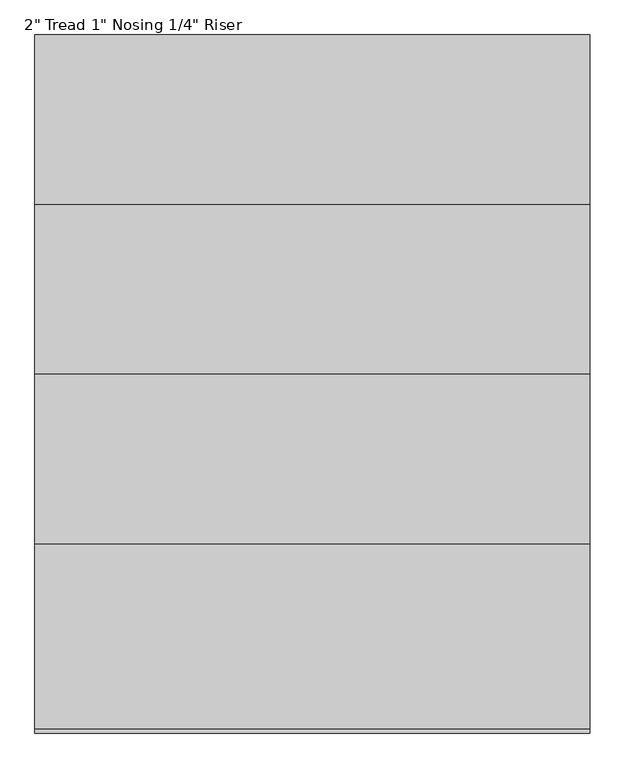
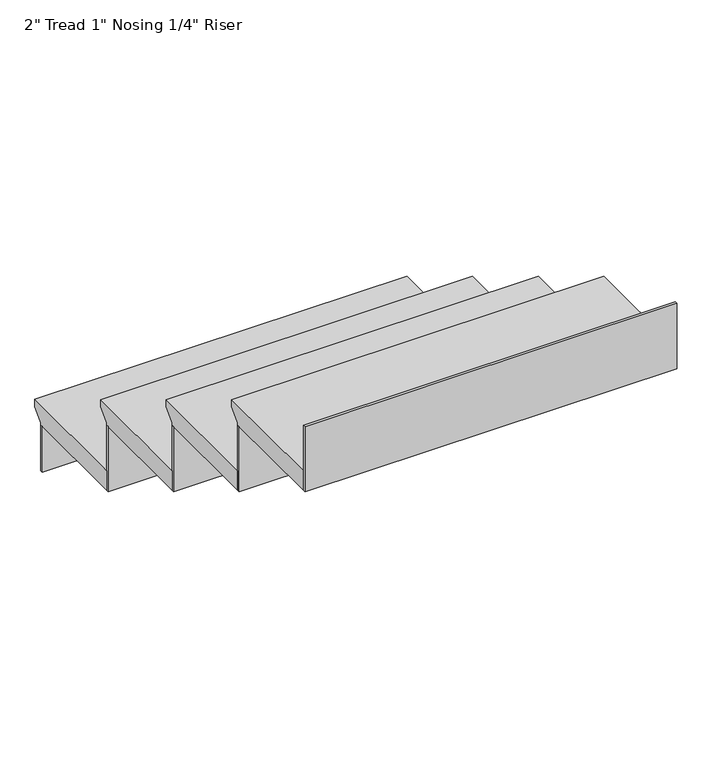
"""IFC4 building model written with IfcOpenShell, lengths in millimetres: stair flight geometry."""

from ifc_helpers import new_model, si_unit, frame, origin, place, context, project, spatial, polyline, outline, extrude, source, transform, mapped, element, save


def stair_flight_987ae6dc(model_context):
    return source(origin(), model_context, "Body", "SweptSolid", [
        extrude(outline(polyline([(618.7061342, 1693.3333333), (923.5061342, 1693.3333333), (923.5061342, 1674.2833333), (898.1061342, 1648.8833333), (898.1061342, 1642.5333333), (618.7061342, 1642.5333333), (618.7061342, 1693.3333333)])), frame((-4563.8448749, 0.0, 0.0), z_axis=(1.0, 0.0, 0.0), x_axis=(0.0, 1.0, 0.0)), (0.0, 0.0, 1.0), 914.4),
        extrude(outline(polyline([(-4563.8448749, 891.7561342), (-4563.8448749, 898.1061342), (-3649.4448749, 898.1061342), (-3649.4448749, 891.7561342), (-4563.8448749, 891.7561342)])), frame((0.0, 0.0, 1524.0), z_axis=(0.0, 0.0, 1.0), x_axis=(1.0, 0.0, 0.0)), (0.0, 0.0, 1.0), 118.5333333),
        extrude(outline(polyline([(-4563.8448749, 612.3561342), (-4563.8448749, 618.7061342), (-3649.4448749, 618.7061342), (-3649.4448749, 612.3561342), (-4563.8448749, 612.3561342)])), frame((0.0, 0.0, 1642.5333333), z_axis=(0.0, 0.0, 1.0), x_axis=(1.0, 0.0, 0.0)), (0.0, 0.0, 1.0), 169.3333333),
        extrude(outline(polyline([(339.3061342, 1862.6666667), (644.1061342, 1862.6666667), (644.1061342, 1843.6166667), (618.7061342, 1818.2166667), (618.7061342, 1811.8666667), (339.3061342, 1811.8666667), (339.3061342, 1862.6666667)])), frame((-4563.8448749, 0.0, 0.0), z_axis=(1.0, 0.0, 0.0), x_axis=(0.0, 1.0, 0.0)), (0.0, 0.0, 1.0), 914.4),
        extrude(outline(polyline([(-4563.8448749, 332.9561342), (-4563.8448749, 339.3061342), (-3649.4448749, 339.3061342), (-3649.4448749, 332.9561342), (-4563.8448749, 332.9561342)])), frame((0.0, 0.0, 1811.8666667), z_axis=(0.0, 0.0, 1.0), x_axis=(1.0, 0.0, 0.0)), (0.0, 0.0, 1.0), 169.3333333),
        extrude(outline(polyline([(59.9061342, 2032.0), (364.7061342, 2032.0), (364.7061342, 2012.95), (339.3061342, 1987.55), (339.3061342, 1981.2), (59.9061342, 1981.2), (59.9061342, 2032.0)])), frame((-4563.8448749, 0.0, 0.0), z_axis=(1.0, 0.0, 0.0), x_axis=(0.0, 1.0, 0.0)), (0.0, 0.0, 1.0), 914.4),
        extrude(outline(polyline([(-4563.8448749, 53.5561342), (-4563.8448749, 59.9061342), (-3649.4448749, 59.9061342), (-3649.4448749, 53.5561342), (-4563.8448749, 53.5561342)])), frame((0.0, 0.0, 1981.2), z_axis=(0.0, 0.0, 1.0), x_axis=(1.0, 0.0, 0.0)), (0.0, 0.0, 1.0), 169.3333333),
        extrude(outline(polyline([(-4563.8448749, -225.8438658), (-4563.8448749, -219.4938658), (-3649.4448749, -219.4938658), (-3649.4448749, -225.8438658), (-4563.8448749, -225.8438658)])), frame((0.0, 0.0, 2150.5333333), z_axis=(0.0, 0.0, 1.0), x_axis=(1.0, 0.0, 0.0)), (0.0, 0.0, 1.0), 169.3333333),
        extrude(outline(polyline([(-219.4938658, 2201.3333333), (85.3061342, 2201.3333333), (85.3061342, 2182.2833333), (59.9061342, 2156.8833333), (59.9061342, 2150.5333333), (-219.4938658, 2150.5333333), (-219.4938658, 2201.3333333)])), frame((-4563.8448749, 0.0, 0.0), z_axis=(1.0, 0.0, 0.0), x_axis=(0.0, 1.0, 0.0)), (0.0, 0.0, 1.0), 914.4),
    ])


if __name__ == "__main__":
    model = new_model("IFC4")
    model_context = context("Model", 3, world=origin())
    ifc_project = project(units=[si_unit("LENGTHUNIT", "METRE", prefix="MILLI")], contexts=[model_context])
    site = spatial("IfcSite", under=ifc_project)
    building = spatial("IfcBuilding", under=site)
    placement = place(None, origin())
    stair_flight_shape = stair_flight_987ae6dc(model_context)
    element("IfcStairFlight", 1, ObjectType="2\" Tread 1\" Nosing 1/4\" Riser", at=placement, inside=building, context=model_context, shape_type="MappedRepresentation", body=[
        mapped(stair_flight_shape, transform((0.0, 0.0, 0.0), x_axis=(1.0, 0.0, 0.0), y_axis=(0.0, 1.0, 0.0), z_axis=(0.0, 0.0, 1.0))),
    ])
    save(model, "model.ifc")
